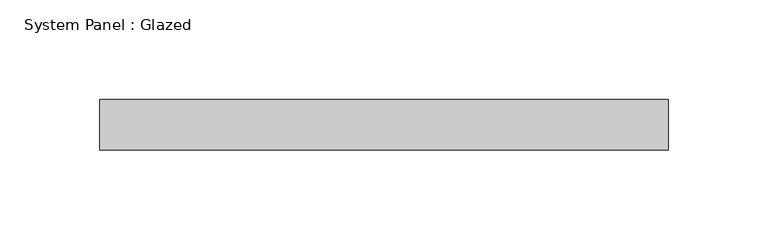
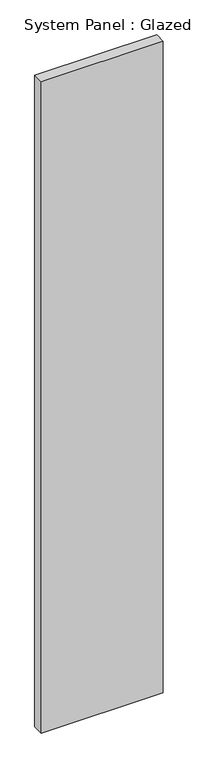
"""IFC4 building model written with IfcOpenShell, lengths in millimetres: plate geometry, System Panel : Glazed."""

from ifc_helpers import new_model, si_unit, origin, origin_with_axes, place, context, project, spatial, polyline, outline, extrude, source, transform, mapped, element, save


def system_panel_glazed_f1a934e3(model_context):
    return source(origin(), model_context, "Body", "SweptSolid", [
        extrude(outline(polyline([(142.875, 19.05), (-142.875, 19.05), (-142.875, 44.45), (142.875, 44.45), (142.875, 19.05)])), origin_with_axes(), (0.0, 0.0, 1.0), 1609.0162259),
    ])


if __name__ == "__main__":
    model = new_model("IFC4")
    model_context = context("Model", 3, world=origin())
    ifc_project = project(units=[si_unit("LENGTHUNIT", "METRE", prefix="MILLI")], contexts=[model_context])
    site = spatial("IfcSite", under=ifc_project)
    building = spatial("IfcBuilding", under=site)
    placement = place(None, origin())
    system_panel_glazed_shape = system_panel_glazed_f1a934e3(model_context)
    element("IfcPlate", 1, ObjectType="System Panel : Glazed", at=placement, inside=building, context=model_context, shape_type="MappedRepresentation", body=[
        mapped(system_panel_glazed_shape, transform((0.0, 0.0, 0.0), x_axis=(1.0, 0.0, 0.0), y_axis=(0.0, 1.0, 0.0), z_axis=(0.0, 0.0, 1.0))),
    ])
    save(model, "model.ifc")

# Revit data of these elements
# Type "System Panel : Glazed"
#   Construction Type Id = "GSP4R"
#   Analytic Construction = "1/8 in Pilkington single glazing"
#   Visual Light Transmittance = 0.9
#   Solar Heat Gain Coefficient = 0.86
#   Heat Transfer Coefficient (U) = 1.18115 BTU/(h·ft²·°F)
#   Define Thermal Properties by = 1
# Element 1 (IfcPlate, "System Panel : Glazed")
#   Materials on its faces: "Glass"
# Materials
#   "Glass": class "Glass", colour RGB 0 128 192, transparency 0.75, Description = "Soda Lime Glass", Cost = 0
